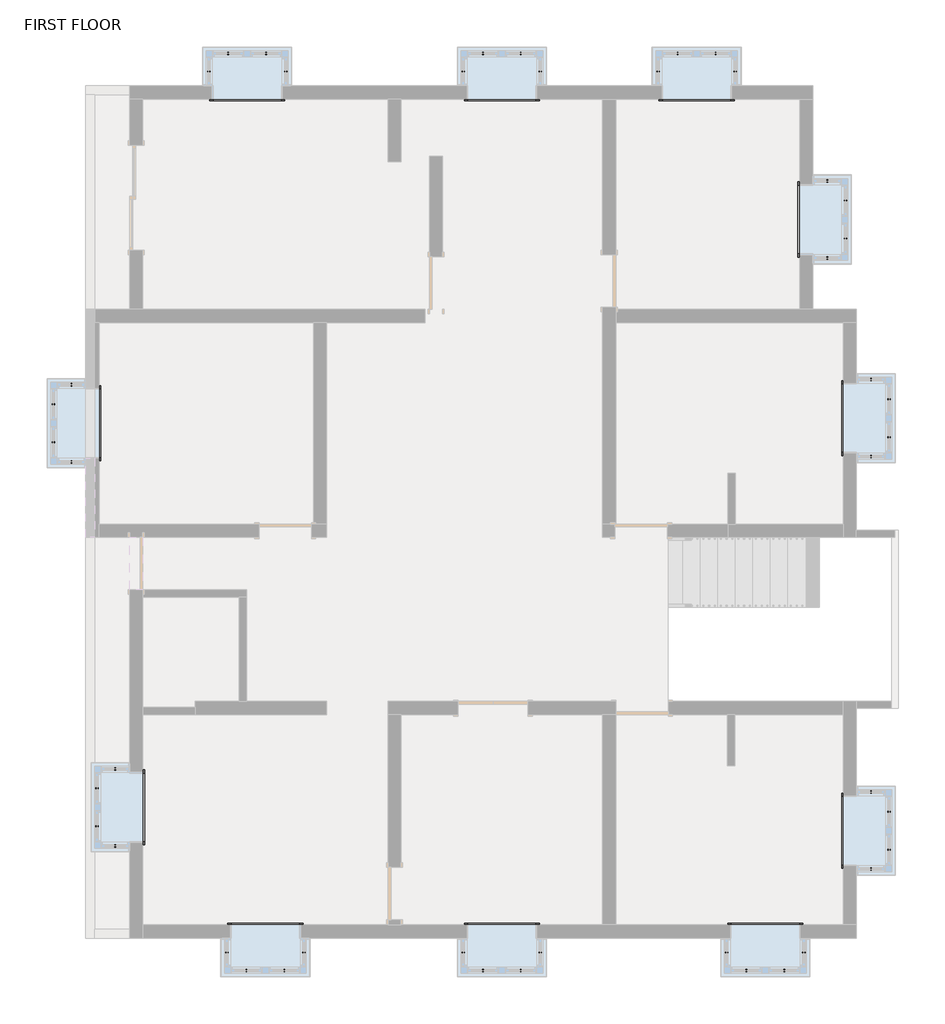
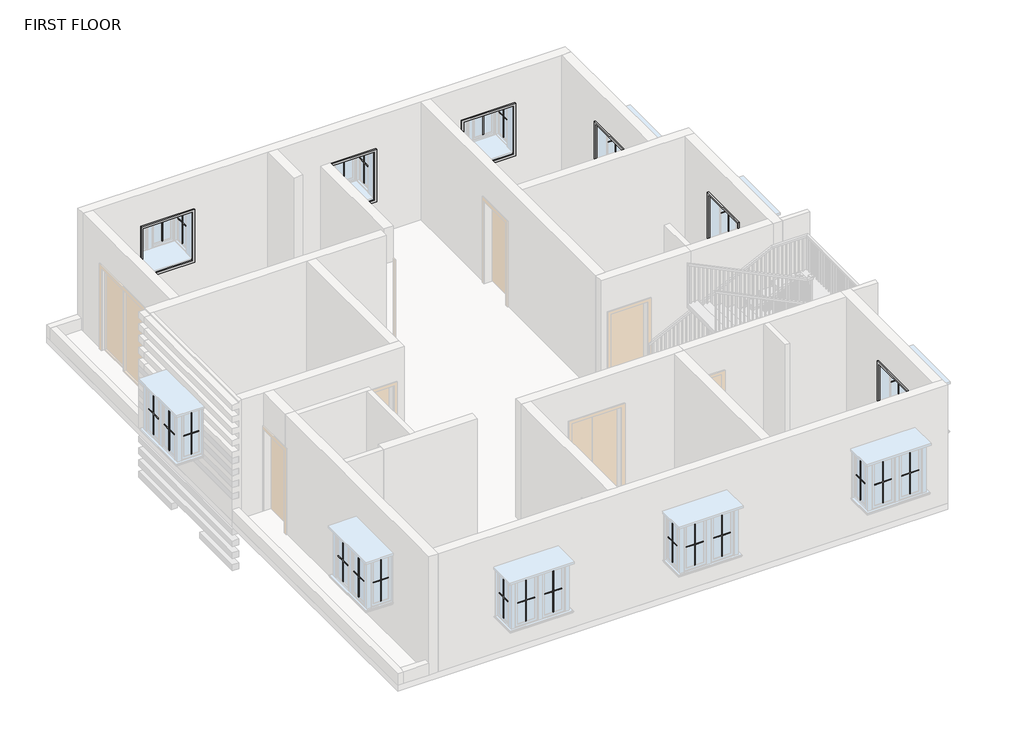
# One storey, part 6 of 6: 55 proxies.
"""IFC4 building model written with IfcOpenShell, lengths in millimetres."""

from ifc_helpers import new_model, si_unit, origin, place, context, project, spatial, transform, mapped, element, save
from components import muntin_pattern_2x2_muntin_pattern_2x2_4aee108e, muntin_pattern_2x2_muntin_pattern_2x2_f03ab90d, muntin_pattern_2x2_muntin_pattern_2x2_eb08c668, trim_window_interior_flat_picture_frame_ace0ae79

model = new_model("IFC4")

# Units and contexts
model_context = context("Model", 3, world=origin())
ifc_project = project(units=[si_unit("LENGTHUNIT", "METRE", prefix="MILLI")], contexts=[model_context])

# Site, building, storey
site = spatial("IfcSite", under=ifc_project)
building = spatial("IfcBuilding", under=site)
storey = spatial("IfcBuildingStorey", under=building, Name="FIRST FLOOR", Elevation=3200.4)

# Proxies
placement = place(None, origin())
muntin_pattern_2x2_muntin_pattern_2x2_shape = muntin_pattern_2x2_muntin_pattern_2x2_4aee108e(model_context)
element("IfcBuildingElementProxy", 1, Name="Muntin Pattern_2x2 : Muntin Pattern_2x2", ObjectType="Muntin Pattern_2x2 : Muntin Pattern_2x2", at=placement, inside=storey, context=model_context, shape_type="MappedRepresentation", body=[
    mapped(muntin_pattern_2x2_muntin_pattern_2x2_shape, transform((6209.1834916, 6075.433346, 4235.45), x_axis=(0.0, -1.0, 0.0), y_axis=(1.0, 0.0, 0.0), z_axis=(0.0, 0.0, 1.0))),
])
element("IfcBuildingElementProxy", 2, Name="Muntin Pattern_2x2 : Muntin Pattern_2x2", ObjectType="Muntin Pattern_2x2 : Muntin Pattern_2x2", at=placement, inside=storey, context=model_context, shape_type="MappedRepresentation", body=[
    mapped(muntin_pattern_2x2_muntin_pattern_2x2_shape, transform((-99.5415084, 8637.658346, 4235.45), x_axis=(1.0, 0.0, 0.0), y_axis=(0.0, 1.0, 0.0), z_axis=(0.0, 0.0, 1.0))),
])
element("IfcBuildingElementProxy", 3, Name="Muntin Pattern_2x2 : Muntin Pattern_2x2", ObjectType="Muntin Pattern_2x2 : Muntin Pattern_2x2", at=placement, inside=storey, context=model_context, shape_type="MappedRepresentation", body=[
    mapped(muntin_pattern_2x2_muntin_pattern_2x2_shape, transform((3291.3584916, 8637.658346, 4235.45), x_axis=(1.0, 0.0, 0.0), y_axis=(0.0, 1.0, 0.0), z_axis=(0.0, 0.0, 1.0))),
])
element("IfcBuildingElementProxy", 4, Name="Muntin Pattern_2x2 : Muntin Pattern_2x2", ObjectType="Muntin Pattern_2x2 : Muntin Pattern_2x2", at=placement, inside=storey, context=model_context, shape_type="MappedRepresentation", body=[
    mapped(muntin_pattern_2x2_muntin_pattern_2x2_shape, transform((-4531.8415084, 8637.658346, 4235.45), x_axis=(1.0, 0.0, 0.0), y_axis=(0.0, 1.0, 0.0), z_axis=(0.0, 0.0, 1.0))),
])
element("IfcBuildingElementProxy", 5, Name="Muntin Pattern_2x2 : Muntin Pattern_2x2", ObjectType="Muntin Pattern_2x2 : Muntin Pattern_2x2", at=placement, inside=storey, context=model_context, shape_type="MappedRepresentation", body=[
    mapped(muntin_pattern_2x2_muntin_pattern_2x2_shape, transform((-7576.6665084, 1871.733346, 4235.45), x_axis=(0.0, 1.0, 0.0), y_axis=(-1.0, 0.0, 0.0), z_axis=(0.0, 0.0, 1.0))),
])
element("IfcBuildingElementProxy", 6, Name="Muntin Pattern_2x2 : Muntin Pattern_2x2", ObjectType="Muntin Pattern_2x2 : Muntin Pattern_2x2", at=placement, inside=storey, context=model_context, shape_type="MappedRepresentation", body=[
    mapped(muntin_pattern_2x2_muntin_pattern_2x2_shape, transform((6971.1834916, 2621.033346, 4235.45), x_axis=(0.0, -1.0, 0.0), y_axis=(1.0, 0.0, 0.0), z_axis=(0.0, 0.0, 1.0))),
])
element("IfcBuildingElementProxy", 7, Name="Muntin Pattern_2x2 : Muntin Pattern_2x2", ObjectType="Muntin Pattern_2x2 : Muntin Pattern_2x2", at=placement, inside=storey, context=model_context, shape_type="MappedRepresentation", body=[
    mapped(muntin_pattern_2x2_muntin_pattern_2x2_shape, transform((-3553.9415084, -7319.891654, 4235.45), x_axis=(-1.0, 0.0, 0.0), y_axis=(0.0, -1.0, 0.0), z_axis=(0.0, 0.0, 1.0))),
])
element("IfcBuildingElementProxy", 8, Name="Muntin Pattern_2x2 : Muntin Pattern_2x2", ObjectType="Muntin Pattern_2x2 : Muntin Pattern_2x2", at=placement, inside=storey, context=model_context, shape_type="MappedRepresentation", body=[
    mapped(muntin_pattern_2x2_muntin_pattern_2x2_shape, transform((5145.5584916, -7319.891654, 4235.45), x_axis=(-1.0, 0.0, 0.0), y_axis=(0.0, -1.0, 0.0), z_axis=(0.0, 0.0, 1.0))),
])
element("IfcBuildingElementProxy", 9, Name="Muntin Pattern_2x2 : Muntin Pattern_2x2", ObjectType="Muntin Pattern_2x2 : Muntin Pattern_2x2", at=placement, inside=storey, context=model_context, shape_type="MappedRepresentation", body=[
    mapped(muntin_pattern_2x2_muntin_pattern_2x2_shape, transform((560.8584916, -7319.891654, 4235.45), x_axis=(-1.0, 0.0, 0.0), y_axis=(0.0, -1.0, 0.0), z_axis=(0.0, 0.0, 1.0))),
])
element("IfcBuildingElementProxy", 10, Name="Muntin Pattern_2x2 : Muntin Pattern_2x2", ObjectType="Muntin Pattern_2x2 : Muntin Pattern_2x2", at=placement, inside=storey, context=model_context, shape_type="MappedRepresentation", body=[
    mapped(muntin_pattern_2x2_muntin_pattern_2x2_shape, transform((-6814.6665084, -4808.466654, 4235.45), x_axis=(0.0, 1.0, 0.0), y_axis=(-1.0, 0.0, 0.0), z_axis=(0.0, 0.0, 1.0))),
])
element("IfcBuildingElementProxy", 11, Name="Muntin Pattern_2x2 : Muntin Pattern_2x2", ObjectType="Muntin Pattern_2x2 : Muntin Pattern_2x2", at=placement, inside=storey, context=model_context, shape_type="MappedRepresentation", body=[
    mapped(muntin_pattern_2x2_muntin_pattern_2x2_shape, transform((6971.1834916, -4554.466654, 4235.45), x_axis=(0.0, -1.0, 0.0), y_axis=(1.0, 0.0, 0.0), z_axis=(0.0, 0.0, 1.0))),
])
muntin_pattern_2x2_muntin_pattern_2x2_2_shape = muntin_pattern_2x2_muntin_pattern_2x2_f03ab90d(model_context)
element("IfcBuildingElementProxy", 12, Name="Muntin Pattern_2x2 : Muntin Pattern_2x2", ObjectType="Muntin Pattern_2x2 : Muntin Pattern_2x2", at=placement, inside=storey, context=model_context, shape_type="MappedRepresentation", body=[
    mapped(muntin_pattern_2x2_muntin_pattern_2x2_2_shape, transform((5894.8584916, 6415.158346, 4235.45), x_axis=(-1.0, 0.0, 0.0), y_axis=(0.0, -1.0, 0.0), z_axis=(0.0, 0.0, 1.0))),
])
element("IfcBuildingElementProxy", 13, Name="Muntin Pattern_2x2 : Muntin Pattern_2x2", ObjectType="Muntin Pattern_2x2 : Muntin Pattern_2x2", at=placement, inside=storey, context=model_context, shape_type="MappedRepresentation", body=[
    mapped(muntin_pattern_2x2_muntin_pattern_2x2_2_shape, transform((5894.8584916, 5075.308346, 4235.45), x_axis=(1.0, 0.0, 0.0), y_axis=(0.0, 1.0, 0.0), z_axis=(0.0, 0.0, 1.0))),
])
element("IfcBuildingElementProxy", 14, Name="Muntin Pattern_2x2 : Muntin Pattern_2x2", ObjectType="Muntin Pattern_2x2 : Muntin Pattern_2x2", at=placement, inside=storey, context=model_context, shape_type="MappedRepresentation", body=[
    mapped(muntin_pattern_2x2_muntin_pattern_2x2_2_shape, transform((-439.2665084, 8323.333346, 4235.45), x_axis=(0.0, -1.0, 0.0), y_axis=(1.0, 0.0, 0.0), z_axis=(0.0, 0.0, 1.0))),
])
element("IfcBuildingElementProxy", 15, Name="Muntin Pattern_2x2 : Muntin Pattern_2x2", ObjectType="Muntin Pattern_2x2 : Muntin Pattern_2x2", at=placement, inside=storey, context=model_context, shape_type="MappedRepresentation", body=[
    mapped(muntin_pattern_2x2_muntin_pattern_2x2_2_shape, transform((900.5834916, 8323.333346, 4235.45), x_axis=(0.0, 1.0, 0.0), y_axis=(-1.0, 0.0, 0.0), z_axis=(0.0, 0.0, 1.0))),
])
element("IfcBuildingElementProxy", 16, Name="Muntin Pattern_2x2 : Muntin Pattern_2x2", ObjectType="Muntin Pattern_2x2 : Muntin Pattern_2x2", at=placement, inside=storey, context=model_context, shape_type="MappedRepresentation", body=[
    mapped(muntin_pattern_2x2_muntin_pattern_2x2_2_shape, transform((2951.6334916, 8323.333346, 4235.45), x_axis=(0.0, -1.0, 0.0), y_axis=(1.0, 0.0, 0.0), z_axis=(0.0, 0.0, 1.0))),
])
element("IfcBuildingElementProxy", 17, Name="Muntin Pattern_2x2 : Muntin Pattern_2x2", ObjectType="Muntin Pattern_2x2 : Muntin Pattern_2x2", at=placement, inside=storey, context=model_context, shape_type="MappedRepresentation", body=[
    mapped(muntin_pattern_2x2_muntin_pattern_2x2_2_shape, transform((4291.4834916, 8323.333346, 4235.45), x_axis=(0.0, 1.0, 0.0), y_axis=(-1.0, 0.0, 0.0), z_axis=(0.0, 0.0, 1.0))),
])
element("IfcBuildingElementProxy", 18, Name="Muntin Pattern_2x2 : Muntin Pattern_2x2", ObjectType="Muntin Pattern_2x2 : Muntin Pattern_2x2", at=placement, inside=storey, context=model_context, shape_type="MappedRepresentation", body=[
    mapped(muntin_pattern_2x2_muntin_pattern_2x2_2_shape, transform((-4871.5665084, 8323.333346, 4235.45), x_axis=(0.0, -1.0, 0.0), y_axis=(1.0, 0.0, 0.0), z_axis=(0.0, 0.0, 1.0))),
])
element("IfcBuildingElementProxy", 19, Name="Muntin Pattern_2x2 : Muntin Pattern_2x2", ObjectType="Muntin Pattern_2x2 : Muntin Pattern_2x2", at=placement, inside=storey, context=model_context, shape_type="MappedRepresentation", body=[
    mapped(muntin_pattern_2x2_muntin_pattern_2x2_2_shape, transform((-3531.7165084, 8323.333346, 4235.45), x_axis=(0.0, 1.0, 0.0), y_axis=(-1.0, 0.0, 0.0), z_axis=(0.0, 0.0, 1.0))),
])
element("IfcBuildingElementProxy", 20, Name="Muntin Pattern_2x2 : Muntin Pattern_2x2", ObjectType="Muntin Pattern_2x2 : Muntin Pattern_2x2", at=placement, inside=storey, context=model_context, shape_type="MappedRepresentation", body=[
    mapped(muntin_pattern_2x2_muntin_pattern_2x2_2_shape, transform((-7262.3415084, 1532.008346, 4235.45), x_axis=(1.0, 0.0, 0.0), y_axis=(0.0, 1.0, 0.0), z_axis=(0.0, 0.0, 1.0))),
])
element("IfcBuildingElementProxy", 21, Name="Muntin Pattern_2x2 : Muntin Pattern_2x2", ObjectType="Muntin Pattern_2x2 : Muntin Pattern_2x2", at=placement, inside=storey, context=model_context, shape_type="MappedRepresentation", body=[
    mapped(muntin_pattern_2x2_muntin_pattern_2x2_2_shape, transform((-7262.3415084, 2871.858346, 4235.45), x_axis=(-1.0, 0.0, 0.0), y_axis=(0.0, -1.0, 0.0), z_axis=(0.0, 0.0, 1.0))),
])
element("IfcBuildingElementProxy", 22, Name="Muntin Pattern_2x2 : Muntin Pattern_2x2", ObjectType="Muntin Pattern_2x2 : Muntin Pattern_2x2", at=placement, inside=storey, context=model_context, shape_type="MappedRepresentation", body=[
    mapped(muntin_pattern_2x2_muntin_pattern_2x2_2_shape, transform((6656.8584916, 2960.758346, 4235.45), x_axis=(-1.0, 0.0, 0.0), y_axis=(0.0, -1.0, 0.0), z_axis=(0.0, 0.0, 1.0))),
])
element("IfcBuildingElementProxy", 23, Name="Muntin Pattern_2x2 : Muntin Pattern_2x2", ObjectType="Muntin Pattern_2x2 : Muntin Pattern_2x2", at=placement, inside=storey, context=model_context, shape_type="MappedRepresentation", body=[
    mapped(muntin_pattern_2x2_muntin_pattern_2x2_2_shape, transform((6656.8584916, 1620.908346, 4235.45), x_axis=(1.0, 0.0, 0.0), y_axis=(0.0, 1.0, 0.0), z_axis=(0.0, 0.0, 1.0))),
])
element("IfcBuildingElementProxy", 24, Name="Muntin Pattern_2x2 : Muntin Pattern_2x2", ObjectType="Muntin Pattern_2x2 : Muntin Pattern_2x2", at=placement, inside=storey, context=model_context, shape_type="MappedRepresentation", body=[
    mapped(muntin_pattern_2x2_muntin_pattern_2x2_2_shape, transform((-3214.2165084, -7005.566654, 4235.45), x_axis=(0.0, 1.0, 0.0), y_axis=(-1.0, 0.0, 0.0), z_axis=(0.0, 0.0, 1.0))),
])
element("IfcBuildingElementProxy", 25, Name="Muntin Pattern_2x2 : Muntin Pattern_2x2", ObjectType="Muntin Pattern_2x2 : Muntin Pattern_2x2", at=placement, inside=storey, context=model_context, shape_type="MappedRepresentation", body=[
    mapped(muntin_pattern_2x2_muntin_pattern_2x2_2_shape, transform((-4554.0665084, -7005.566654, 4235.45), x_axis=(0.0, -1.0, 0.0), y_axis=(1.0, 0.0, 0.0), z_axis=(0.0, 0.0, 1.0))),
])
element("IfcBuildingElementProxy", 26, Name="Muntin Pattern_2x2 : Muntin Pattern_2x2", ObjectType="Muntin Pattern_2x2 : Muntin Pattern_2x2", at=placement, inside=storey, context=model_context, shape_type="MappedRepresentation", body=[
    mapped(muntin_pattern_2x2_muntin_pattern_2x2_2_shape, transform((5485.2834916, -7005.566654, 4235.45), x_axis=(0.0, 1.0, 0.0), y_axis=(-1.0, 0.0, 0.0), z_axis=(0.0, 0.0, 1.0))),
])
element("IfcBuildingElementProxy", 27, Name="Muntin Pattern_2x2 : Muntin Pattern_2x2", ObjectType="Muntin Pattern_2x2 : Muntin Pattern_2x2", at=placement, inside=storey, context=model_context, shape_type="MappedRepresentation", body=[
    mapped(muntin_pattern_2x2_muntin_pattern_2x2_2_shape, transform((4145.4334916, -7005.566654, 4235.45), x_axis=(0.0, -1.0, 0.0), y_axis=(1.0, 0.0, 0.0), z_axis=(0.0, 0.0, 1.0))),
])
element("IfcBuildingElementProxy", 28, Name="Muntin Pattern_2x2 : Muntin Pattern_2x2", ObjectType="Muntin Pattern_2x2 : Muntin Pattern_2x2", at=placement, inside=storey, context=model_context, shape_type="MappedRepresentation", body=[
    mapped(muntin_pattern_2x2_muntin_pattern_2x2_2_shape, transform((900.5834916, -7005.566654, 4235.45), x_axis=(0.0, 1.0, 0.0), y_axis=(-1.0, 0.0, 0.0), z_axis=(0.0, 0.0, 1.0))),
])
element("IfcBuildingElementProxy", 29, Name="Muntin Pattern_2x2 : Muntin Pattern_2x2", ObjectType="Muntin Pattern_2x2 : Muntin Pattern_2x2", at=placement, inside=storey, context=model_context, shape_type="MappedRepresentation", body=[
    mapped(muntin_pattern_2x2_muntin_pattern_2x2_2_shape, transform((-439.2665084, -7005.566654, 4235.45), x_axis=(0.0, -1.0, 0.0), y_axis=(1.0, 0.0, 0.0), z_axis=(0.0, 0.0, 1.0))),
])
element("IfcBuildingElementProxy", 30, Name="Muntin Pattern_2x2 : Muntin Pattern_2x2", ObjectType="Muntin Pattern_2x2 : Muntin Pattern_2x2", at=placement, inside=storey, context=model_context, shape_type="MappedRepresentation", body=[
    mapped(muntin_pattern_2x2_muntin_pattern_2x2_2_shape, transform((-6500.3415084, -5148.191654, 4235.45), x_axis=(1.0, 0.0, 0.0), y_axis=(0.0, 1.0, 0.0), z_axis=(0.0, 0.0, 1.0))),
])
element("IfcBuildingElementProxy", 31, Name="Muntin Pattern_2x2 : Muntin Pattern_2x2", ObjectType="Muntin Pattern_2x2 : Muntin Pattern_2x2", at=placement, inside=storey, context=model_context, shape_type="MappedRepresentation", body=[
    mapped(muntin_pattern_2x2_muntin_pattern_2x2_2_shape, transform((-6500.3415084, -3808.341654, 4235.45), x_axis=(-1.0, 0.0, 0.0), y_axis=(0.0, -1.0, 0.0), z_axis=(0.0, 0.0, 1.0))),
])
element("IfcBuildingElementProxy", 32, Name="Muntin Pattern_2x2 : Muntin Pattern_2x2", ObjectType="Muntin Pattern_2x2 : Muntin Pattern_2x2", at=placement, inside=storey, context=model_context, shape_type="MappedRepresentation", body=[
    mapped(muntin_pattern_2x2_muntin_pattern_2x2_2_shape, transform((6656.8584916, -4214.741654, 4235.45), x_axis=(-1.0, 0.0, 0.0), y_axis=(0.0, -1.0, 0.0), z_axis=(0.0, 0.0, 1.0))),
])
element("IfcBuildingElementProxy", 33, Name="Muntin Pattern_2x2 : Muntin Pattern_2x2", ObjectType="Muntin Pattern_2x2 : Muntin Pattern_2x2", at=placement, inside=storey, context=model_context, shape_type="MappedRepresentation", body=[
    mapped(muntin_pattern_2x2_muntin_pattern_2x2_2_shape, transform((6656.8584916, -5554.591654, 4235.45), x_axis=(1.0, 0.0, 0.0), y_axis=(0.0, 1.0, 0.0), z_axis=(0.0, 0.0, 1.0))),
])
muntin_pattern_2x2_muntin_pattern_2x2_3_shape = muntin_pattern_2x2_muntin_pattern_2x2_eb08c668(model_context)
element("IfcBuildingElementProxy", 34, Name="Muntin Pattern_2x2 : Muntin Pattern_2x2", ObjectType="Muntin Pattern_2x2 : Muntin Pattern_2x2", at=placement, inside=storey, context=model_context, shape_type="MappedRepresentation", body=[
    mapped(muntin_pattern_2x2_muntin_pattern_2x2_3_shape, transform((6209.1834916, 5415.033346, 4235.45), x_axis=(0.0, 1.0, 0.0), y_axis=(-1.0, 0.0, 0.0), z_axis=(0.0, 0.0, 1.0))),
])
element("IfcBuildingElementProxy", 35, Name="Muntin Pattern_2x2 : Muntin Pattern_2x2", ObjectType="Muntin Pattern_2x2 : Muntin Pattern_2x2", at=placement, inside=storey, context=model_context, shape_type="MappedRepresentation", body=[
    mapped(muntin_pattern_2x2_muntin_pattern_2x2_3_shape, transform((560.8584916, 8637.658346, 4235.45), x_axis=(-1.0, 0.0, 0.0), y_axis=(0.0, -1.0, 0.0), z_axis=(0.0, 0.0, 1.0))),
])
element("IfcBuildingElementProxy", 36, Name="Muntin Pattern_2x2 : Muntin Pattern_2x2", ObjectType="Muntin Pattern_2x2 : Muntin Pattern_2x2", at=placement, inside=storey, context=model_context, shape_type="MappedRepresentation", body=[
    mapped(muntin_pattern_2x2_muntin_pattern_2x2_3_shape, transform((3951.7584916, 8637.658346, 4235.45), x_axis=(-1.0, 0.0, 0.0), y_axis=(0.0, -1.0, 0.0), z_axis=(0.0, 0.0, 1.0))),
])
element("IfcBuildingElementProxy", 37, Name="Muntin Pattern_2x2 : Muntin Pattern_2x2", ObjectType="Muntin Pattern_2x2 : Muntin Pattern_2x2", at=placement, inside=storey, context=model_context, shape_type="MappedRepresentation", body=[
    mapped(muntin_pattern_2x2_muntin_pattern_2x2_3_shape, transform((-3871.4415084, 8637.658346, 4235.45), x_axis=(-1.0, 0.0, 0.0), y_axis=(0.0, -1.0, 0.0), z_axis=(0.0, 0.0, 1.0))),
])
element("IfcBuildingElementProxy", 38, Name="Muntin Pattern_2x2 : Muntin Pattern_2x2", ObjectType="Muntin Pattern_2x2 : Muntin Pattern_2x2", at=placement, inside=storey, context=model_context, shape_type="MappedRepresentation", body=[
    mapped(muntin_pattern_2x2_muntin_pattern_2x2_3_shape, transform((-7576.6665084, 2532.133346, 4235.45), x_axis=(0.0, -1.0, 0.0), y_axis=(1.0, 0.0, 0.0), z_axis=(0.0, 0.0, 1.0))),
])
element("IfcBuildingElementProxy", 39, Name="Muntin Pattern_2x2 : Muntin Pattern_2x2", ObjectType="Muntin Pattern_2x2 : Muntin Pattern_2x2", at=placement, inside=storey, context=model_context, shape_type="MappedRepresentation", body=[
    mapped(muntin_pattern_2x2_muntin_pattern_2x2_3_shape, transform((6971.1834916, 1960.633346, 4235.45), x_axis=(0.0, 1.0, 0.0), y_axis=(-1.0, 0.0, 0.0), z_axis=(0.0, 0.0, 1.0))),
])
element("IfcBuildingElementProxy", 40, Name="Muntin Pattern_2x2 : Muntin Pattern_2x2", ObjectType="Muntin Pattern_2x2 : Muntin Pattern_2x2", at=placement, inside=storey, context=model_context, shape_type="MappedRepresentation", body=[
    mapped(muntin_pattern_2x2_muntin_pattern_2x2_3_shape, transform((-4214.3415084, -7319.891654, 4235.45), x_axis=(1.0, 0.0, 0.0), y_axis=(0.0, 1.0, 0.0), z_axis=(0.0, 0.0, 1.0))),
])
element("IfcBuildingElementProxy", 41, Name="Muntin Pattern_2x2 : Muntin Pattern_2x2", ObjectType="Muntin Pattern_2x2 : Muntin Pattern_2x2", at=placement, inside=storey, context=model_context, shape_type="MappedRepresentation", body=[
    mapped(muntin_pattern_2x2_muntin_pattern_2x2_3_shape, transform((4485.1584916, -7319.891654, 4235.45), x_axis=(1.0, 0.0, 0.0), y_axis=(0.0, 1.0, 0.0), z_axis=(0.0, 0.0, 1.0))),
])
element("IfcBuildingElementProxy", 42, Name="Muntin Pattern_2x2 : Muntin Pattern_2x2", ObjectType="Muntin Pattern_2x2 : Muntin Pattern_2x2", at=placement, inside=storey, context=model_context, shape_type="MappedRepresentation", body=[
    mapped(muntin_pattern_2x2_muntin_pattern_2x2_3_shape, transform((-99.5415084, -7319.891654, 4235.45), x_axis=(1.0, 0.0, 0.0), y_axis=(0.0, 1.0, 0.0), z_axis=(0.0, 0.0, 1.0))),
])
element("IfcBuildingElementProxy", 43, Name="Muntin Pattern_2x2 : Muntin Pattern_2x2", ObjectType="Muntin Pattern_2x2 : Muntin Pattern_2x2", at=placement, inside=storey, context=model_context, shape_type="MappedRepresentation", body=[
    mapped(muntin_pattern_2x2_muntin_pattern_2x2_3_shape, transform((-6814.6665084, -4148.066654, 4235.45), x_axis=(0.0, -1.0, 0.0), y_axis=(1.0, 0.0, 0.0), z_axis=(0.0, 0.0, 1.0))),
])
element("IfcBuildingElementProxy", 44, Name="Muntin Pattern_2x2 : Muntin Pattern_2x2", ObjectType="Muntin Pattern_2x2 : Muntin Pattern_2x2", at=placement, inside=storey, context=model_context, shape_type="MappedRepresentation", body=[
    mapped(muntin_pattern_2x2_muntin_pattern_2x2_3_shape, transform((6971.1834916, -5214.866654, 4235.45), x_axis=(0.0, 1.0, 0.0), y_axis=(-1.0, 0.0, 0.0), z_axis=(0.0, 0.0, 1.0))),
])
trim_window_interior_flat_picture_frame_shape = trim_window_interior_flat_picture_frame_ace0ae79(model_context)
element("IfcBuildingElementProxy", 45, Name="Trim-Window-Interior-Flat : Picture Frame", ObjectType="Trim-Window-Interior-Flat : Picture Frame", at=placement, inside=storey, context=model_context, shape_type="MappedRepresentation", body=[
    mapped(trim_window_interior_flat_picture_frame_shape, transform((5412.2584916, 5745.233346, 5384.8), x_axis=(0.0, -1.0, 0.0), y_axis=(0.0, 0.0, 1.0), z_axis=(-1.0, 0.0, 0.0))),
])
element("IfcBuildingElementProxy", 46, Name="Trim-Window-Interior-Flat : Picture Frame", ObjectType="Trim-Window-Interior-Flat : Picture Frame", at=placement, inside=storey, context=model_context, shape_type="MappedRepresentation", body=[
    mapped(trim_window_interior_flat_picture_frame_shape, transform((230.6584916, 7840.733346, 5384.8), x_axis=(1.0, 0.0, 0.0), y_axis=(0.0, 0.0, 1.0), z_axis=(0.0, -1.0, 0.0))),
])
element("IfcBuildingElementProxy", 47, Name="Trim-Window-Interior-Flat : Picture Frame", ObjectType="Trim-Window-Interior-Flat : Picture Frame", at=placement, inside=storey, context=model_context, shape_type="MappedRepresentation", body=[
    mapped(trim_window_interior_flat_picture_frame_shape, transform((3621.5584916, 7840.733346, 5384.8), x_axis=(1.0, 0.0, 0.0), y_axis=(0.0, 0.0, 1.0), z_axis=(0.0, -1.0, 0.0))),
])
element("IfcBuildingElementProxy", 48, Name="Trim-Window-Interior-Flat : Picture Frame", ObjectType="Trim-Window-Interior-Flat : Picture Frame", at=placement, inside=storey, context=model_context, shape_type="MappedRepresentation", body=[
    mapped(trim_window_interior_flat_picture_frame_shape, transform((-4201.6415084, 7840.733346, 5384.8), x_axis=(1.0, 0.0, 0.0), y_axis=(0.0, 0.0, 1.0), z_axis=(0.0, -1.0, 0.0))),
])
element("IfcBuildingElementProxy", 49, Name="Trim-Window-Interior-Flat : Picture Frame", ObjectType="Trim-Window-Interior-Flat : Picture Frame", at=placement, inside=storey, context=model_context, shape_type="MappedRepresentation", body=[
    mapped(trim_window_interior_flat_picture_frame_shape, transform((-6779.7415084, 2201.933346, 5384.8), x_axis=(0.0, 1.0, 0.0), y_axis=(0.0, 0.0, 1.0), z_axis=(1.0, 0.0, 0.0))),
])
element("IfcBuildingElementProxy", 50, Name="Trim-Window-Interior-Flat : Picture Frame", ObjectType="Trim-Window-Interior-Flat : Picture Frame", at=placement, inside=storey, context=model_context, shape_type="MappedRepresentation", body=[
    mapped(trim_window_interior_flat_picture_frame_shape, transform((6174.2584916, 2290.833346, 5384.8), x_axis=(0.0, -1.0, 0.0), y_axis=(0.0, 0.0, 1.0), z_axis=(-1.0, 0.0, 0.0))),
])
element("IfcBuildingElementProxy", 51, Name="Trim-Window-Interior-Flat : Picture Frame", ObjectType="Trim-Window-Interior-Flat : Picture Frame", at=placement, inside=storey, context=model_context, shape_type="MappedRepresentation", body=[
    mapped(trim_window_interior_flat_picture_frame_shape, transform((-3884.1415084, -6522.966654, 5384.8), x_axis=(-1.0, 0.0, 0.0), y_axis=(0.0, 0.0, 1.0), z_axis=(0.0, 1.0, 0.0))),
])
element("IfcBuildingElementProxy", 52, Name="Trim-Window-Interior-Flat : Picture Frame", ObjectType="Trim-Window-Interior-Flat : Picture Frame", at=placement, inside=storey, context=model_context, shape_type="MappedRepresentation", body=[
    mapped(trim_window_interior_flat_picture_frame_shape, transform((4815.3584916, -6522.966654, 5384.8), x_axis=(-1.0, 0.0, 0.0), y_axis=(0.0, 0.0, 1.0), z_axis=(0.0, 1.0, 0.0))),
])
element("IfcBuildingElementProxy", 53, Name="Trim-Window-Interior-Flat : Picture Frame", ObjectType="Trim-Window-Interior-Flat : Picture Frame", at=placement, inside=storey, context=model_context, shape_type="MappedRepresentation", body=[
    mapped(trim_window_interior_flat_picture_frame_shape, transform((230.6584916, -6522.966654, 5384.8), x_axis=(-1.0, 0.0, 0.0), y_axis=(0.0, 0.0, 1.0), z_axis=(0.0, 1.0, 0.0))),
])
element("IfcBuildingElementProxy", 54, Name="Trim-Window-Interior-Flat : Picture Frame", ObjectType="Trim-Window-Interior-Flat : Picture Frame", at=placement, inside=storey, context=model_context, shape_type="MappedRepresentation", body=[
    mapped(trim_window_interior_flat_picture_frame_shape, transform((-6017.7415084, -4478.266654, 5384.8), x_axis=(0.0, 1.0, 0.0), y_axis=(0.0, 0.0, 1.0), z_axis=(1.0, 0.0, 0.0))),
])
element("IfcBuildingElementProxy", 55, Name="Trim-Window-Interior-Flat : Picture Frame", ObjectType="Trim-Window-Interior-Flat : Picture Frame", at=placement, inside=storey, context=model_context, shape_type="MappedRepresentation", body=[
    mapped(trim_window_interior_flat_picture_frame_shape, transform((6174.2584916, -4884.666654, 5384.8), x_axis=(0.0, -1.0, 0.0), y_axis=(0.0, 0.0, 1.0), z_axis=(-1.0, 0.0, 0.0))),
])

save(model, "model.ifc")

# Revit data of these elements
# Type "Muntin Pattern_2x2 : Muntin Pattern_2x2"
#   Width [instance default] = 4' - 0"
#   Thickness = 0' - 0 1/2"
#   Height [instance default] = 4' - 0"
#   Distance = 0' - 0 3/4"
#   Interior Material [instance default] = none
#   Exterior Material [instance default] = none
#   Default Elevation = 0
# Type "Trim-Window-Interior-Flat : Picture Frame"
#   Trim Thickness_Picture Frame = 0' - 1 1/4"
#   Trim Width = 0' - 2 1/4"
#   Trim Thickness_with Sill = 0' - 0 3/4"
#   Sill Thickness = 0' - 1 1/4"
#   Opening Width [instance default] = 2' - 0"
#   Opening Height [instance default] = 3' - 0"
#   Default Elevation = 4' - 0"
#   Sill = no
#   Picture Frame = yes
#   Trim Material [instance default] = none
# Elements 1, 2, 3, 4, 5, 6, 7, 8, 9, 10, 11, 34, 35, 36, 37, 38, 39, 40, 41, 42, 43, 44 (IfcBuildingElementProxy, "Muntin Pattern_2x2 : Muntin Pattern_2x2")
#   Width = 1' - 4 1/2"
#   Height = 3' - 6 1/2"
#   Interior Material = Wood - Stained
#   Exterior Material = Clad - White
#   Phase Created = New Construction
#   Materials on its faces: "Clad - White", "Wood - Stained"
# Elements 12, 13, 14, 15, 16, 17, 18, 19, 20, 21, 22, 23, 24, 25, 26, 27, 28, 29, 30, 31, 32, 33 (IfcBuildingElementProxy, "Muntin Pattern_2x2 : Muntin Pattern_2x2")
#   Width = 1' - 2 1/2"
#   Height = 3' - 6 1/2"
#   Interior Material = Wood - Stained
#   Exterior Material = Clad - White
#   Phase Created = New Construction
#   Materials on its faces: "Clad - White", "Wood - Stained"
# Elements 45, 46, 47, 48, 49, 50, 51, 52, 53, 54, 55 (IfcBuildingElementProxy, "Trim-Window-Interior-Flat : Picture Frame")
#   Opening Width = 4' - 0"
#   Opening Height = 4' - 2"
#   Trim Material = Wood - Stained
#   Phase Created = New Construction
#   Materials on its faces: "Wood - Stained"
# Materials
#   "Clad - White": class "Wood", colour RGB 242 242 238, transparency 0, Cost = 0
#   "Wood - Stained": class "Wood", colour RGB 224 178 126, transparency 0, Cost = 0
